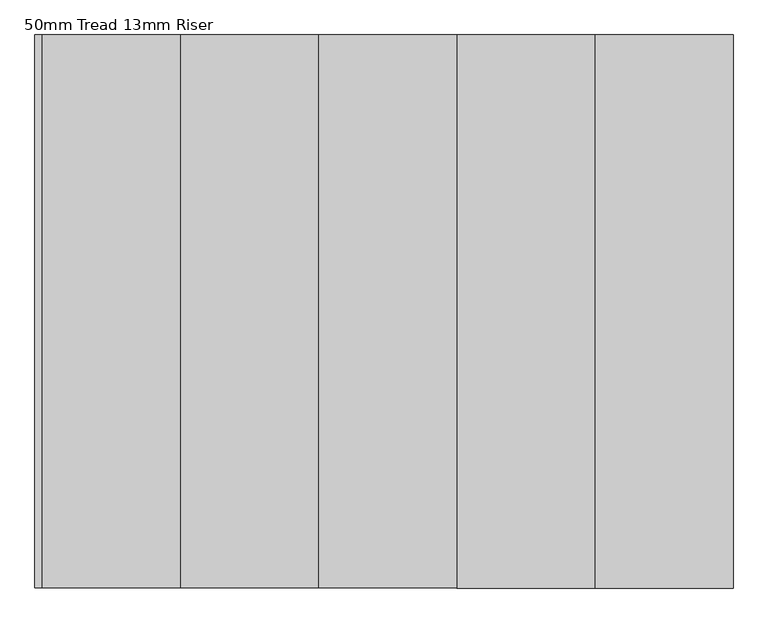
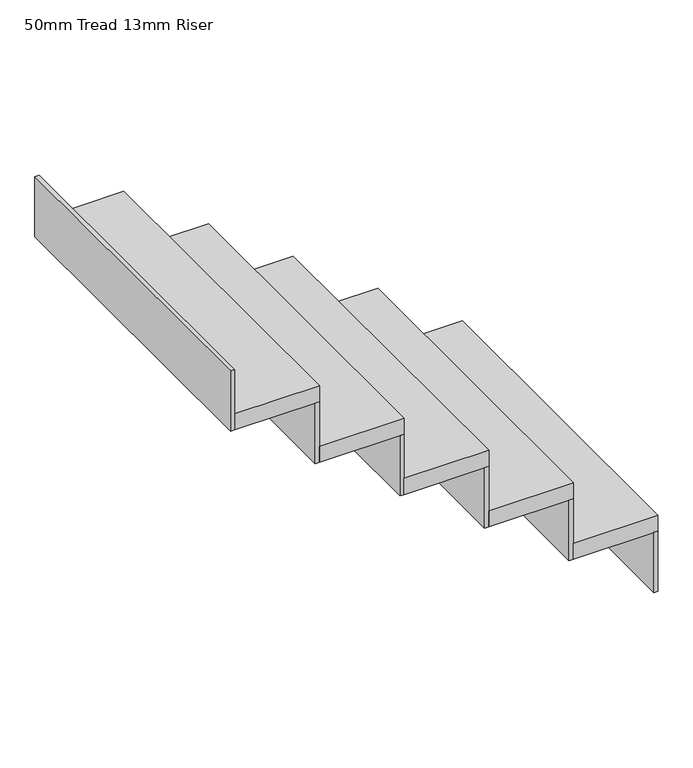
"""IFC4 building model written with IfcOpenShell, lengths in millimetres: stair flight geometry, 50mm Tread 13mm Riser."""

from ifc_helpers import new_model, si_unit, frame, origin, place, context, project, spatial, polyline, outline, extrude, source, transform, mapped, element, save


def stair_flight_50mm_tread_13mm_riser_ab5ce904(model_context):
    return source(origin(), model_context, "Body", "SweptSolid", [
        extrude(outline(polyline([(-10480.6794909, -3251.1360696), (-10468.1794909, -3251.1360696), (-10468.1794909, -4251.1618509), (-10480.6794909, -4251.1618509), (-10480.6794909, -3251.1360696)])), frame((0.0, 0.0, 11622.0470588), z_axis=(0.0, 0.0, 1.0), x_axis=(1.0, 0.0, 0.0)), (0.0, 0.0, 1.0), 188.2588235),
        extrude(outline(polyline([(-10718.1794909, -4251.1618509), (-10718.1794909, -3251.1360696), (-10468.1794909, -3251.1360696), (-10468.1794909, -4251.1618509), (-10718.1794909, -4251.1618509)])), frame((0.0, 0.0, 11810.3058824), z_axis=(0.0, 0.0, 1.0), x_axis=(1.0, 0.0, 0.0)), (0.0, 0.0, 1.0), 50.0),
        extrude(outline(polyline([(-10730.6794909, -3251.1360696), (-10718.1794909, -3251.1360696), (-10718.1794909, -4251.1618509), (-10730.6794909, -4251.1618509), (-10730.6794909, -3251.1360696)])), frame((0.0, 0.0, 11810.3058824), z_axis=(0.0, 0.0, 1.0), x_axis=(1.0, 0.0, 0.0)), (0.0, 0.0, 1.0), 188.2588235),
        extrude(outline(polyline([(-10968.1794909, -4251.1618509), (-10968.1794909, -3251.1360696), (-10718.1794909, -3251.1360696), (-10718.1794909, -4251.1618509), (-10968.1794909, -4251.1618509)])), frame((0.0, 0.0, 11998.5647059), z_axis=(0.0, 0.0, 1.0), x_axis=(1.0, 0.0, 0.0)), (0.0, 0.0, 1.0), 50.0),
        extrude(outline(polyline([(-10980.6794909, -3251.1360696), (-10968.1794909, -3251.1360696), (-10968.1794909, -4251.1618509), (-10980.6794909, -4251.1618509), (-10980.6794909, -3251.1360696)])), frame((0.0, 0.0, 11998.5647059), z_axis=(0.0, 0.0, 1.0), x_axis=(1.0, 0.0, 0.0)), (0.0, 0.0, 1.0), 188.2588235),
        extrude(outline(polyline([(-11218.1794909, -4251.1618509), (-11218.1794909, -3251.1360696), (-10968.1794909, -3251.1360696), (-10968.1794909, -4251.1618509), (-11218.1794909, -4251.1618509)])), frame((0.0, 0.0, 12186.8235294), z_axis=(0.0, 0.0, 1.0), x_axis=(1.0, 0.0, 0.0)), (0.0, 0.0, 1.0), 50.0),
        extrude(outline(polyline([(-11230.6794909, -3251.1360696), (-11218.1794909, -3251.1360696), (-11218.1794909, -4251.1618509), (-11230.6794909, -4251.1618509), (-11230.6794909, -3251.1360696)])), frame((0.0, 0.0, 12186.8235294), z_axis=(0.0, 0.0, 1.0), x_axis=(1.0, 0.0, 0.0)), (0.0, 0.0, 1.0), 188.2588235),
        extrude(outline(polyline([(-11468.1794909, -4251.1618509), (-11468.1794909, -3251.1360696), (-11218.1794909, -3251.1360696), (-11218.1794909, -4251.1618509), (-11468.1794909, -4251.1618509)])), frame((0.0, 0.0, 12375.0823529), z_axis=(0.0, 0.0, 1.0), x_axis=(1.0, 0.0, 0.0)), (0.0, 0.0, 1.0), 50.0),
        extrude(outline(polyline([(-11480.6794909, -3251.1360696), (-11468.1794909, -3251.1360696), (-11468.1794909, -4251.1618509), (-11480.6794909, -4251.1618509), (-11480.6794909, -3251.1360696)])), frame((0.0, 0.0, 12375.0823529), z_axis=(0.0, 0.0, 1.0), x_axis=(1.0, 0.0, 0.0)), (0.0, 0.0, 1.0), 188.2588235),
        extrude(outline(polyline([(-11730.6794909, -3251.1360696), (-11718.1794909, -3251.1360696), (-11718.1794909, -4251.1618509), (-11730.6794909, -4251.1618509), (-11730.6794909, -3251.1360696)])), frame((0.0, 0.0, 12563.3411765), z_axis=(0.0, 0.0, 1.0), x_axis=(1.0, 0.0, 0.0)), (0.0, 0.0, 1.0), 188.2588235),
        extrude(outline(polyline([(-11718.1794909, -4251.1618509), (-11718.1794909, -3251.1360696), (-11468.1794909, -3251.1360696), (-11468.1794909, -4251.1618509), (-11718.1794909, -4251.1618509)])), frame((0.0, 0.0, 12563.3411765), z_axis=(0.0, 0.0, 1.0), x_axis=(1.0, 0.0, 0.0)), (0.0, 0.0, 1.0), 50.0),
    ])


if __name__ == "__main__":
    model = new_model("IFC4")
    model_context = context("Model", 3, world=origin())
    ifc_project = project(units=[si_unit("LENGTHUNIT", "METRE", prefix="MILLI")], contexts=[model_context])
    site = spatial("IfcSite", under=ifc_project)
    building = spatial("IfcBuilding", under=site)
    placement = place(None, origin())
    stair_flight_50mm_tread_13mm_riser_shape = stair_flight_50mm_tread_13mm_riser_ab5ce904(model_context)
    element("IfcStairFlight", 1, ObjectType="50mm Tread 13mm Riser", at=placement, inside=building, context=model_context, shape_type="MappedRepresentation", body=[
        mapped(stair_flight_50mm_tread_13mm_riser_shape, transform((0.0, 0.0, 0.0), x_axis=(1.0, 0.0, 0.0), y_axis=(0.0, 1.0, 0.0), z_axis=(0.0, 0.0, 1.0))),
    ])
    save(model, "model.ifc")
